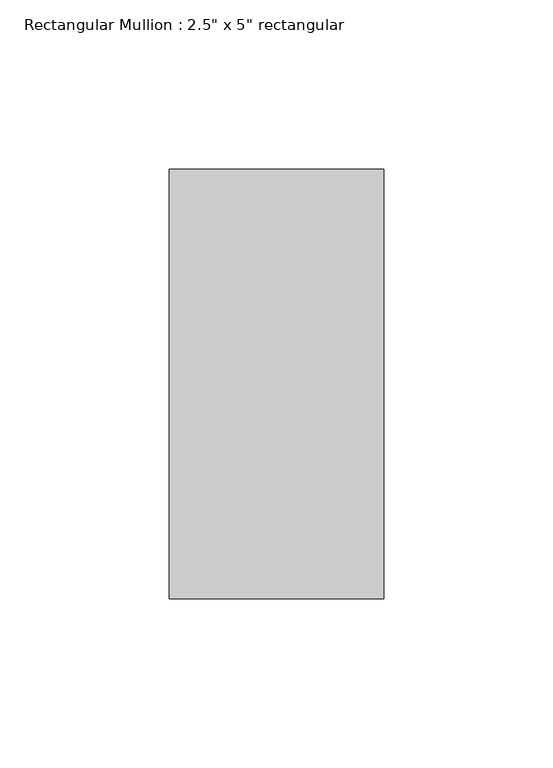
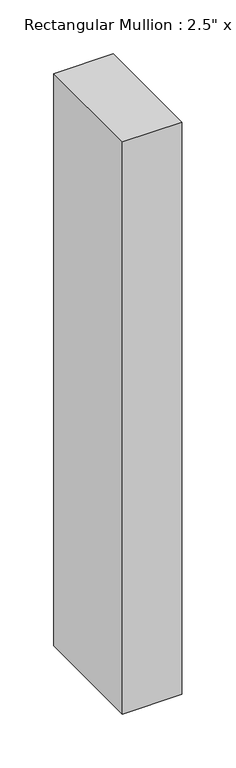
"""IFC4 building model written with IfcOpenShell, lengths in millimetres: member geometry."""

from ifc_helpers import new_model, si_unit, frame, origin, place, context, project, spatial, polyline, outline, extrude, source, transform, mapped, element, save


def member_5215b92c(model_context):
    return source(origin(), model_context, "Body", "SweptSolid", [
        extrude(outline(polyline([(0.0, 63.5), (0.0, -63.5), (-63.5, -63.5), (-63.5, 63.5), (0.0, 63.5)])), frame((0.0, 0.0, -647.7), z_axis=(0.0, 0.0, 1.0), x_axis=(1.0, 0.0, 0.0)), (0.0, 0.0, 1.0), 647.7),
    ])


if __name__ == "__main__":
    model = new_model("IFC4")
    model_context = context("Model", 3, world=origin())
    ifc_project = project(units=[si_unit("LENGTHUNIT", "METRE", prefix="MILLI")], contexts=[model_context])
    site = spatial("IfcSite", under=ifc_project)
    building = spatial("IfcBuilding", under=site)
    placement = place(None, origin())
    member_shape = member_5215b92c(model_context)
    element("IfcMember", 1, ObjectType="Rectangular Mullion : 2.5\" x 5\" rectangular", at=placement, inside=building, context=model_context, shape_type="MappedRepresentation", body=[
        mapped(member_shape, transform((0.0, 0.0, 0.0), x_axis=(1.0, 0.0, 0.0), y_axis=(0.0, 1.0, 0.0), z_axis=(0.0, 0.0, 1.0))),
    ])
    save(model, "model.ifc")

# Revit data of these elements
# Type "Rectangular Mullion : 2.5\" x 5\" rectangular"
#   built-in parameter 1007304 = 0.416667 (stored number, unit not read)
#   built-in parameter 1007301 = 0.104167 (stored number, unit not read)
#   built-in parameter 1007300 = 0.104167 (stored number, unit not read)
